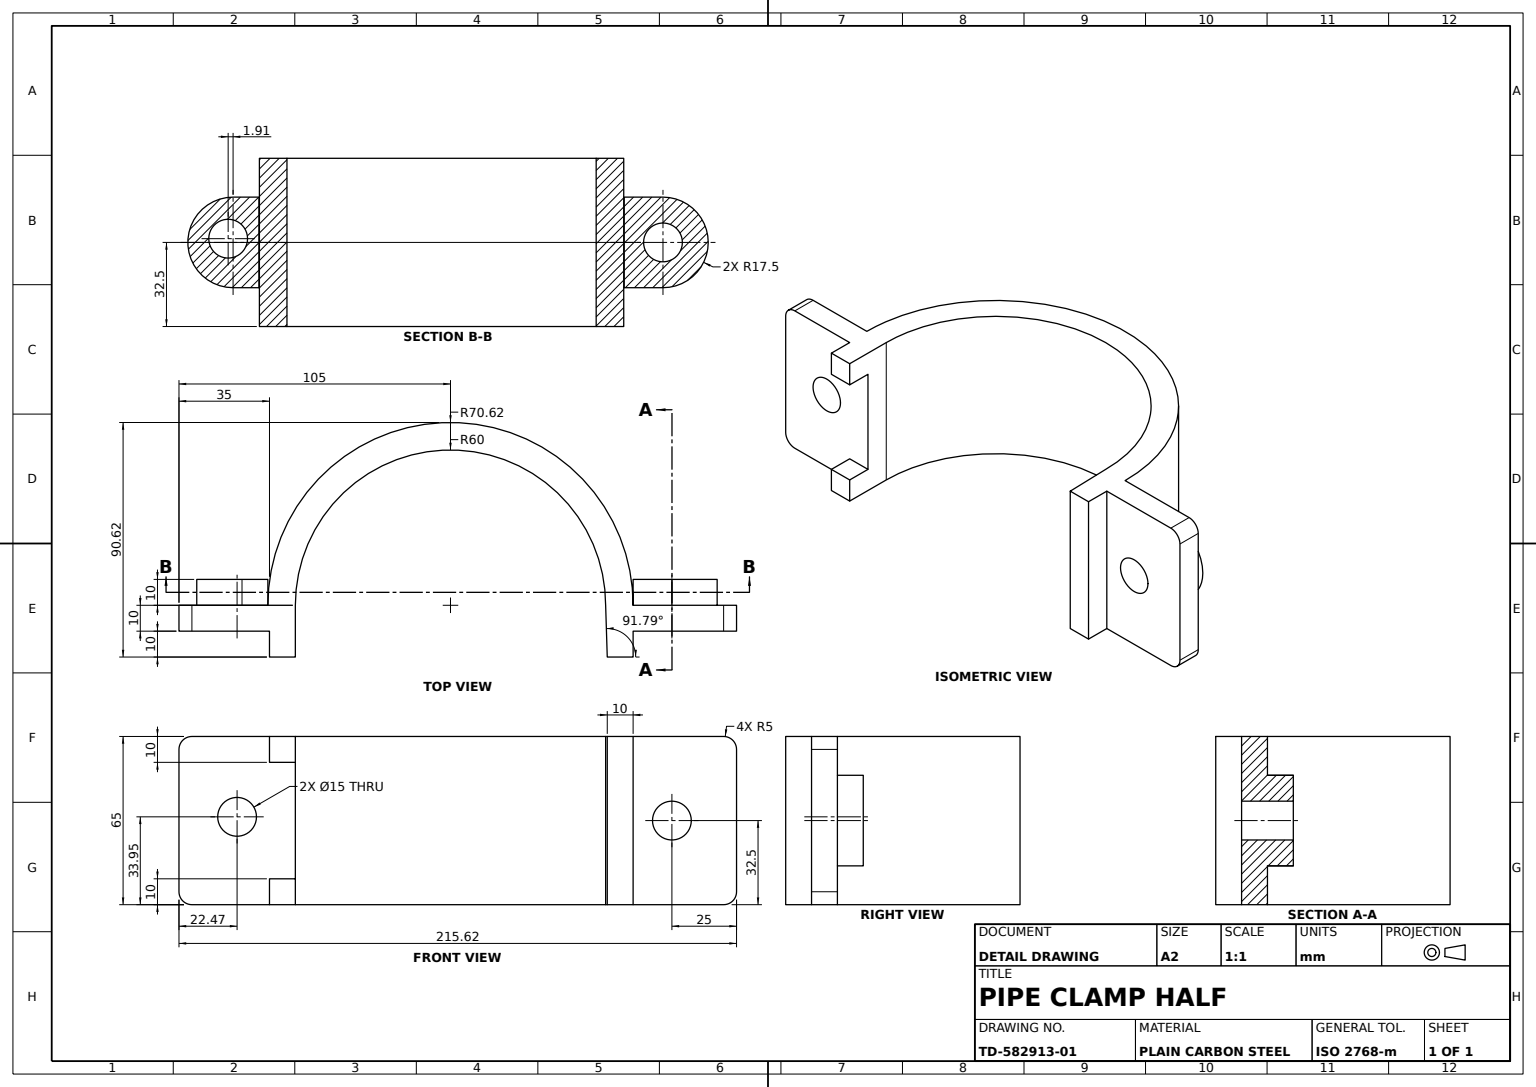
from build123d import *

# Parameters (mm, degrees)
FLANGE_STEP_A_DEPTH  = 10
FLANGE_RIB_SKETCH_W  = 10
FLANGE_RIB_SKETCH_H  = 10
FLANGE_RIB_DEPTH     = 10
CLAMP_BAND_DEPTH     = 65
FLANGE_STEP_B_DEPTH  = 10
FLANGE_WEB_DEPTH     = 65
MOUNTING_LUG_1_DEPTH = 10
MOUNTING_LUG_2_DEPTH = 10
BOLT_HOLE_1_SKETCH_R = 7.5
BOLT_HOLE_1_15_DEPTH = 20
BOLT_HOLE_2_SKETCH_R = 7.5
BOLT_HOLE_2_15_DEPTH = 20


with BuildPart() as part:
    # Flange Step A Sketch → Flange Step A (new body)
    with BuildSketch(Plane.XY):
        with BuildLine():
            Line((0, 10), (-40, 10))
            ThreePointArc((-40, 10), (-43.535533906, 11.464466094), (-45, 15))
            Line((-45, 15), (-45, 70))
            ThreePointArc((-45, 70), (-43.535533906, 73.535533906), (-40, 75))
            Line((-40, 75), (0, 75))
            Line((0, 75), (0, 10))
        make_face()
    extrude(amount=FLANGE_STEP_A_DEPTH)

    # Flange Rib Sketch → Flange Rib (add)
    with BuildSketch(Plane.XY.offset(10)):
        with Locations((-5, 70)):
            Rectangle(FLANGE_RIB_SKETCH_W, FLANGE_RIB_SKETCH_H)
        with Locations((-5, 15)):
            Rectangle(FLANGE_RIB_SKETCH_W, FLANGE_RIB_SKETCH_H)
    extrude(amount=FLANGE_RIB_DEPTH)

    # Clamp Band Sketch → Clamp Band (add)
    with BuildSketch(Plane(origin=(0, 75, 0), x_dir=(1, 0, 0), z_dir=(0, 1, 0))):
        with BuildLine():
            Line((-10.624085248, 0), (0, 0))
            ThreePointArc((0, 0), (60, 60), (120, 0))
            Line((120, 0), (130.624085248, 0))
            ThreePointArc((130.624085248, 0), (60, 70.624085248), (-10.624085248, 0))
        make_face()
    extrude(amount=-CLAMP_BAND_DEPTH)



with BuildPart() as body_2:
    # Flange Step B Sketch → Flange Step B (new body)
    with BuildSketch(Plane.XY):
        with BuildLine():
            Line((130.624085248, 75), (165.624085248, 75))
            ThreePointArc((165.624085248, 75), (169.159619153, 73.535533906), (170.624085248, 70))
            Line((170.624085248, 70), (170.624085248, 15))
            ThreePointArc((170.624085248, 15), (169.159619153, 11.464466094), (165.624085248, 10))
            Line((165.624085248, 10), (130.624085248, 10))
            Line((130.624085248, 10), (130.624085248, 75))
        make_face()
    extrude(amount=FLANGE_STEP_B_DEPTH)


with BuildPart() as part_1:
    add(part.part)

    add(body_2.part)  # Flange Web merges body 2
    # Flange Web Sketch → Flange Web (add)
    with BuildSketch(Plane(origin=(0, 75, 0), x_dir=(1, 0, 0), z_dir=(0, 1, 0))):
        Polygon((130.624085248, 0), (130.624085248, -20), (120.624085248, -20), (120, 0), align=None)
    extrude(amount=-FLANGE_WEB_DEPTH)

    # Mounting Lug 1 Sketch → Mounting Lug 1 (add)
    with BuildSketch(Plane(origin=(0, 0, 0), x_dir=(-1, 0, 0), z_dir=(0, 0, -1))):
        with BuildLine():
            Line((-130.624085248, 60), (-145.624085248, 60))
            ThreePointArc((-145.624085248, 60), (-163.124085248, 42.5), (-145.624085248, 25))
            Line((-145.624085248, 25), (-130.624085248, 25))
            Line((-130.624085248, 25), (-130.624085248, 60))
        make_face()
    extrude(amount=MOUNTING_LUG_1_DEPTH)

    # Mounting Lug 2 Sketch → Mounting Lug 2 (add)
    with BuildSketch(Plane(origin=(0, 0, 0), x_dir=(-1, 0, 0), z_dir=(0, 0, -1))):
        with BuildLine():
            Line((10.624085248, 60), (10.624085248, 25))
            Line((10.624085248, 25), (20.624085248, 25))
            ThreePointArc((20.624085248, 25), (38.124085248, 42.5), (20.624085248, 60))
            Line((20.624085248, 60), (10.624085248, 60))
        make_face()
    extrude(amount=MOUNTING_LUG_2_DEPTH)

    # Bolt Hole 1 Sketch → Bolt Hole 1 Ø15 (cut)
    with BuildSketch(Plane(origin=(0, 0, -10), x_dir=(-1, 0, 0), z_dir=(0, 0, -1))):
        with Locations((-145.624085248, 42.5)):
            Circle(BOLT_HOLE_1_SKETCH_R)
    extrude(amount=-BOLT_HOLE_1_15_DEPTH, mode=Mode.SUBTRACT)

    # Bolt Hole 2 Sketch → Bolt Hole 2 Ø15 (cut)
    with BuildSketch(Plane(origin=(0, 0, -10), x_dir=(-1, 0, 0), z_dir=(0, 0, -1))):
        with Locations((22.530823522, 43.946489257)):
            Circle(BOLT_HOLE_2_SKETCH_R)
    extrude(amount=-BOLT_HOLE_2_15_DEPTH, mode=Mode.SUBTRACT)


solid = part_1.part
